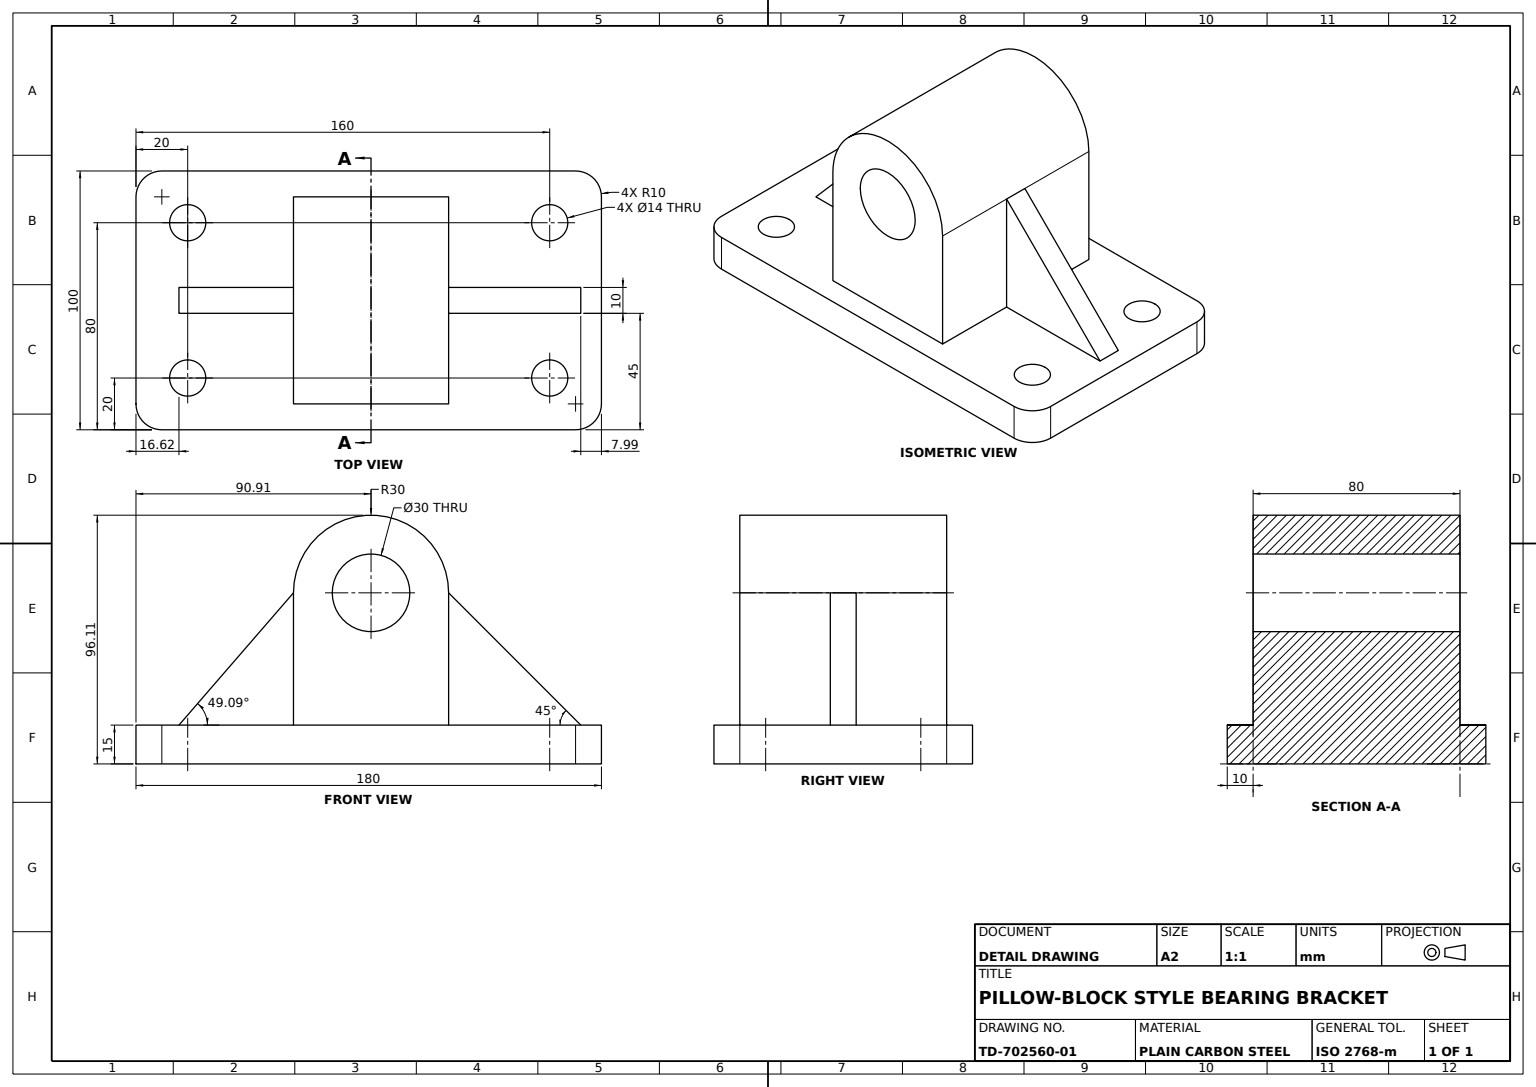
from build123d import *

# Parameters (mm, degrees)
BASE_PLATE_SKETCH_W             = 180
BASE_PLATE_SKETCH_H             = 15
BASE_PLATE_DEPTH                = 100
BEARING_UPRIGHT_SKETCH_R        = 30
BEARING_UPRIGHT_SKETCH_R_2      = 15
BEARING_UPRIGHT_DEPTH           = 40
UPRIGHT_BLOCK_SKETCH_W          = 60
UPRIGHT_BLOCK_SKETCH_H          = 51.105876717
UPRIGHT_BLOCK_DEPTH             = 40
BEARING_START                   = -80
BEARING_BORE_SKETCH_R           = 15
BEARING_BORE_DEPTH              = 80
SUPPORT_RIB_A_REACH             = 212.087
SUPPORT_RIB_A_SKETCH_WALL_W     = 492.173009792
SUPPORT_RIB_A_SKETCH_WALL_H     = 10
SUPPORT_RIB_B_REACH             = 212.087
SUPPORT_RIB_B_SKETCH_WALL_W     = 492.173009792
SUPPORT_RIB_B_SKETCH_WALL_H     = 10
BASE_PLATE_CUT_A_SKETCH_R       = 7
BASE_PLATE_CUT_A_DEPTH          = 80
BASE_PLATE_CUT_B_SKETCH_R       = 7
BASE_PLATE_CUT_B_DEPTH          = 222.310106498
BASE_PLATE_CORNER_FILLETS_R10_R = 10


with BuildPart() as part:
    # Base Plate Sketch → Base Plate (new body)
    with BuildSketch(Plane.XY):
        with Locations((90, 7.5)):
            Rectangle(BASE_PLATE_SKETCH_W, BASE_PLATE_SKETCH_H)
    extrude(amount=BASE_PLATE_DEPTH)



with BuildPart() as body_2:
    # Bearing Upright Sketch → Bearing Upright (new, symmetric)
    with BuildSketch(Plane.XY.offset(50)):
        with Locations((90.90588176, 66.105876717)):
            Circle(BEARING_UPRIGHT_SKETCH_R)
        with Locations((90.90588176, 66.105876717)):
            Circle(BEARING_UPRIGHT_SKETCH_R_2, mode=Mode.SUBTRACT)
    extrude(amount=BEARING_UPRIGHT_DEPTH, both=True)


with BuildPart() as part_1:
    add(part.part)

    add(body_2.part)  # Upright Block merges body 2
    # Upright Block Sketch → Upright Block (add, symmetric)
    with BuildSketch(Plane.XY.offset(50)):
        with Locations((90.90588176, 40.552938359)):
            Rectangle(UPRIGHT_BLOCK_SKETCH_W, UPRIGHT_BLOCK_SKETCH_H)
    extrude(amount=UPRIGHT_BLOCK_DEPTH, both=True)

    # Bearing Bore Sketch → Bearing Bore (cut)
    with BuildSketch(Plane.XY.offset(90).offset(BEARING_START)):
        with Locations((90.90588176, 66.105876717)):
            Circle(BEARING_BORE_SKETCH_R)
    extrude(amount=BEARING_BORE_DEPTH, mode=Mode.SUBTRACT)

    # Support Rib A Sketch wall → Support Rib A (add, up to next)
    with BuildSketch(Plane(origin=(37.986107853, 39.654336798, 50), x_dir=(-0.654850683055, -0.755758283383, 0), z_dir=(0.755758283383, -0.654850683055, 0)), mode=Mode.PRIVATE) as support_rib_a_sk1:
        Rectangle(SUPPORT_RIB_A_SKETCH_WALL_W, SUPPORT_RIB_A_SKETCH_WALL_H)
    support_rib_a_tool1 = extrude(support_rib_a_sk1.sketch, amount=SUPPORT_RIB_A_REACH, mode=Mode.PRIVATE) - part_1.part
    add(support_rib_a_tool1.solids().sort_by_distance((37.986107853, 39.654336798, 50))[0])

    # Support Rib B Sketch wall → Support Rib B (add, up to next)
    with BuildSketch(Plane(origin=(145.654619102, 41.357139375, 50), x_dir=(0.707106781187, -0.707106781187, 0), z_dir=(0.707106781187, 0.707106781187, 0)), mode=Mode.PRIVATE) as support_rib_b_sk1:
        Rectangle(SUPPORT_RIB_B_SKETCH_WALL_W, SUPPORT_RIB_B_SKETCH_WALL_H)
    support_rib_b_tool1 = extrude(support_rib_b_sk1.sketch, amount=-SUPPORT_RIB_B_REACH, mode=Mode.PRIVATE) - part_1.part
    add(support_rib_b_tool1.solids().sort_by_distance((145.654619102, 41.357139375, 50))[0])

    # Base Plate Cut A Sketch → Base Plate Cut A (cut)
    with BuildSketch(Plane(origin=(0, 15, 0), x_dir=(1, 0, 0), z_dir=(0, 1, 0))):
        with Locations(Location((20, -20, 0), (0, 0, 270))):
            Circle(BASE_PLATE_CUT_A_SKETCH_R)
    extrude(amount=-BASE_PLATE_CUT_A_DEPTH, mode=Mode.SUBTRACT)

    # Base Plate Cut B Sketch → Base Plate Cut B (cut, through all)
    with BuildSketch(Plane(origin=(0, 15, 0), x_dir=(1, 0, 0), z_dir=(0, 1, 0))):
        with Locations(Location((160, -20, 0), (0, 0, 270))):
            Circle(BASE_PLATE_CUT_B_SKETCH_R)
        with Locations(Location((160, -80, 0), (0, 0, 270))):
            Circle(BASE_PLATE_CUT_B_SKETCH_R)
        with Locations(Location((20, -80, 0), (0, 0, 270))):
            Circle(BASE_PLATE_CUT_B_SKETCH_R)
    extrude(amount=-BASE_PLATE_CUT_B_DEPTH, mode=Mode.SUBTRACT)

    # Base Plate Corner Fillets R10
    base_plate_corner_fillets_r10_edges = [part_1.edges().sort_by_distance(p)[0] for p in [
        (180, 7.5, 100),
        (0, 7.5, 100),
        (180, 7.5, 0),
        (0, 7.5, 0),
    ]]
    fillet(base_plate_corner_fillets_r10_edges, radius=BASE_PLATE_CORNER_FILLETS_R10_R)


solid = part_1.part
